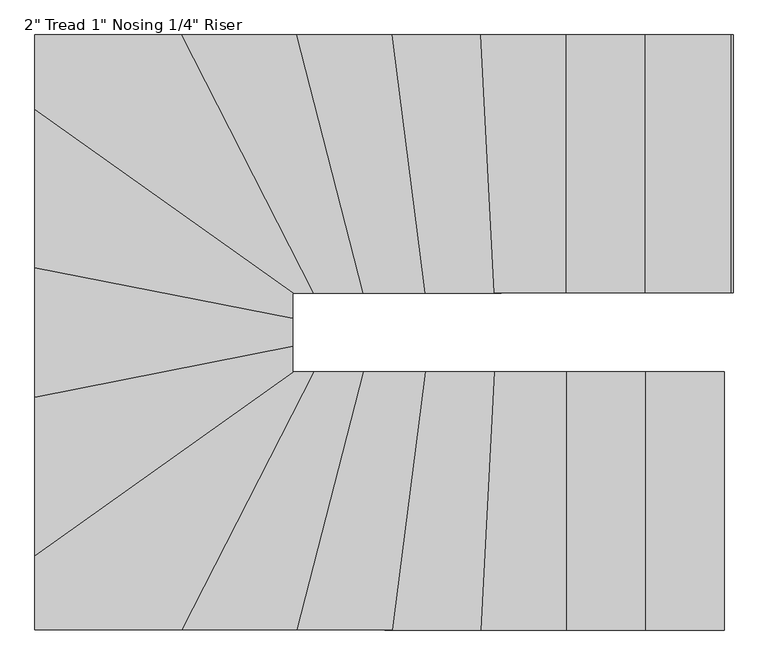
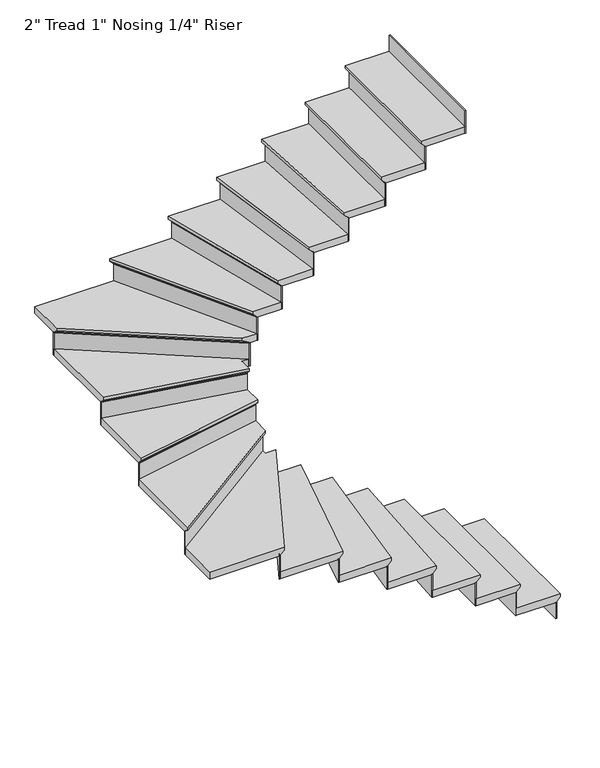
"""IFC4 building model written with IfcOpenShell, lengths in millimetres: stair flight geometry."""

from ifc_helpers import new_model, si_unit, origin, place, context, project, spatial, faceted_brep, source, transform, mapped, element, save


def stair_flight_6e6a5ea5(model_context):
    return source(origin(), model_context, "Body", "Brep", [
        faceted_brep([(-1660.1449167, -345.7070853, 150.2833333), (-1660.1449167, -345.7070853, 169.3333333), (-1660.1449167, -1260.1070853, 169.3333333), (-1660.1449167, -1260.1070853, 150.2833333), (-1685.5449167, -345.7070853, 124.8833333), (-1685.5449167, -1260.1070853, 124.8833333), (-1964.9449167, -345.7070853, 169.3333333), (-1964.9449167, -1260.1070853, 169.3333333), (-1685.5449167, -1260.1070853, 118.5333333), (-1964.9449167, -1260.1070853, 118.5333333), (-1964.9449167, -345.7070853, 118.5333333), (-1685.5449167, -345.7070853, 118.5333333)], [[[0, 1, 2, 3]], [[4, 0, 3, 5]], [[2, 1, 6, 7]], [[8, 9, 10, 11]], [[2, 7, 9, 8, 5, 3]], [[8, 11, 4, 5]], [[6, 1, 0, 4, 11, 10]], [[7, 6, 10, 9]]]),
        faceted_brep([(-1685.5449167, -345.7070853, 118.5333333), (-1685.5449167, -345.7070853, 0.0), (-1691.8949167, -345.7070853, 0.0), (-1691.8949167, -345.7070853, 118.5333333), (-1685.5449167, -1260.1070853, 118.5333333), (-1691.8949167, -1260.1070853, 118.5333333), (-1691.8949167, -1260.1070853, 0.0), (-1685.5449167, -1260.1070853, 0.0)], [[[0, 1, 2, 3]], [[4, 5, 6, 7]], [[1, 0, 4, 7]], [[2, 1, 7, 6]], [[3, 2, 6, 5]], [[0, 3, 5, 4]]]),
        faceted_brep([(-1964.9449167, -345.7070853, 287.8666667), (-1964.9449167, -345.7070853, 118.5333333), (-1971.2949167, -345.7070853, 118.5333333), (-1971.2949167, -345.7070853, 287.8666667), (-1964.9449167, -1260.1070853, 287.8666667), (-1971.2949167, -1260.1070853, 287.8666667), (-1971.2949167, -1260.1070853, 118.5333333), (-1964.9449167, -1260.1070853, 118.5333333)], [[[0, 1, 2, 3]], [[4, 5, 6, 7]], [[1, 0, 4, 7]], [[2, 1, 7, 6]], [[3, 2, 6, 5]], [[0, 3, 5, 4]]]),
        faceted_brep([(-1939.5449167, -1260.1070853, 338.6666667), (-1939.5449167, -345.7070853, 338.6666667), (-2244.3449167, -345.7070853, 338.6666667), (-2244.3449167, -1260.1070853, 338.6666667), (-1964.9449167, -1260.1070853, 287.8666667), (-2244.3449167, -1260.1070853, 287.8666667), (-2244.3449167, -345.7070853, 287.8666667), (-1964.9449167, -345.7070853, 287.8666667), (-1964.9449167, -1260.1070853, 294.2166667), (-1939.5449167, -1260.1070853, 319.6166667), (-1964.9449167, -345.7070853, 294.2166667), (-1939.5449167, -345.7070853, 319.6166667)], [[[0, 1, 2, 3]], [[4, 5, 6, 7]], [[0, 3, 5, 4, 8, 9]], [[4, 7, 10, 8]], [[2, 1, 11, 10, 7, 6]], [[3, 2, 6, 5]], [[11, 1, 0, 9]], [[10, 11, 9, 8]]]),
        faceted_brep([(-2244.3449167, -345.7070853, 457.2), (-2244.3449167, -345.7070853, 287.8666667), (-2250.6949167, -345.7070853, 287.8666667), (-2250.6949167, -345.7070853, 457.2), (-2244.3449167, -1260.1070853, 457.2), (-2250.6949167, -1260.1070853, 457.2), (-2250.6949167, -1260.1070853, 287.8666667), (-2244.3449167, -1260.1070853, 287.8666667)], [[[0, 1, 2, 3]], [[4, 5, 6, 7]], [[1, 0, 4, 7]], [[2, 1, 7, 6]], [[3, 2, 6, 5]], [[0, 3, 5, 4]]]),
        faceted_brep([(-2218.9449167, -1260.1070853, 508.0), (-2218.9449167, -345.7070853, 508.0), (-2500.0120781, -345.7070853, 508.0), (-2547.5463485, -1260.1070853, 508.0), (-2244.3449167, -1260.1070853, 457.2), (-2547.5463485, -1260.1070853, 457.2), (-2500.0120781, -345.7070853, 457.2), (-2244.3449167, -345.7070853, 457.2), (-2244.3449167, -1260.1070853, 463.55), (-2218.9449167, -1260.1070853, 488.95), (-2244.3449167, -345.7070853, 463.55), (-2218.9449167, -345.7070853, 488.95)], [[[0, 1, 2, 3]], [[4, 5, 6, 7]], [[0, 3, 5, 4, 8, 9]], [[4, 7, 10, 8]], [[2, 1, 11, 10, 7, 6]], [[3, 2, 6, 5]], [[11, 1, 0, 9]], [[10, 11, 9, 8]]]),
        faceted_brep([(-2500.0120781, -345.7070853, 626.5333333), (-2500.0120781, -345.7070853, 457.2), (-2506.3706523, -345.7070853, 457.2), (-2506.3706523, -345.7070853, 626.5333333), (-2547.5463485, -1260.1070853, 626.5333333), (-2553.9049227, -1260.1070853, 626.5333333), (-2553.9049227, -1260.1070853, 457.2), (-2547.5463485, -1260.1070853, 457.2)], [[[0, 1, 2, 3]], [[4, 5, 6, 7]], [[1, 0, 4, 7]], [[2, 1, 7, 6]], [[3, 2, 6, 5]], [[0, 3, 5, 4]]]),
        faceted_brep([(-2522.1120519, -1260.1070853, 677.3333333), (-2474.5777815, -345.7070853, 677.3333333), (-2744.178778, -345.7070853, 677.3333333), (-2862.5348296, -1260.1070853, 677.3333333), (-2547.5463485, -1260.1070853, 626.5333333), (-2862.5348296, -1260.1070853, 626.5333333), (-2744.178778, -345.7070853, 626.5333333), (-2500.0120781, -345.7070853, 626.5333333), (-2547.5463485, -1260.1070853, 632.8833333), (-2522.1120519, -1260.1070853, 658.2833333), (-2500.0120781, -345.7070853, 632.8833333), (-2474.5777815, -345.7070853, 658.2833333)], [[[0, 1, 2, 3]], [[4, 5, 6, 7]], [[0, 3, 5, 4, 8, 9]], [[4, 7, 10, 8]], [[2, 1, 11, 10, 7, 6]], [[3, 2, 6, 5]], [[11, 1, 0, 9]], [[10, 11, 9, 8]]]),
        faceted_brep([(-2744.178778, -345.7070853, 795.8666667), (-2744.178778, -345.7070853, 626.5333333), (-2750.5817497, -345.7070853, 626.5333333), (-2750.5817497, -345.7070853, 795.8666667), (-2862.5348296, -1260.1070853, 795.8666667), (-2868.9378014, -1260.1070853, 795.8666667), (-2868.9378014, -1260.1070853, 626.5333333), (-2862.5348296, -1260.1070853, 626.5333333)], [[[0, 1, 2, 3]], [[4, 5, 6, 7]], [[1, 0, 4, 7]], [[2, 1, 7, 6]], [[3, 2, 6, 5]], [[0, 3, 5, 4]]]),
        faceted_brep([(-2836.9229425, -1260.1070853, 846.6666667), (-2718.5668908, -345.7070853, 846.6666667), (-2965.8060004, -345.7070853, 846.6666667), (-3200.9364478, -1260.1070853, 846.6666667), (-2862.5348296, -1260.1070853, 795.8666667), (-3200.9364478, -1260.1070853, 795.8666667), (-2965.8060004, -345.7070853, 795.8666667), (-2744.178778, -345.7070853, 795.8666667), (-2862.5348296, -1260.1070853, 802.2166667), (-2836.9229425, -1260.1070853, 827.6166667), (-2744.178778, -345.7070853, 802.2166667), (-2718.5668908, -345.7070853, 827.6166667)], [[[0, 1, 2, 3]], [[4, 5, 6, 7]], [[0, 3, 5, 4, 8, 9]], [[4, 7, 10, 8]], [[2, 1, 11, 10, 7, 6]], [[3, 2, 6, 5]], [[11, 1, 0, 9]], [[10, 11, 9, 8]]]),
        faceted_brep([(-2965.8060004, -345.7070853, 965.2), (-2965.8060004, -345.7070853, 795.8666667), (-2972.3625773, -345.7070853, 795.8666667), (-2972.3625773, -345.7070853, 965.2), (-3200.9364478, -1260.1070853, 965.2), (-3207.4930247, -1260.1070853, 965.2), (-3207.4930247, -1260.1070853, 795.8666667), (-3200.9364478, -1260.1070853, 795.8666667)], [[[0, 1, 2, 3]], [[4, 5, 6, 7]], [[1, 0, 4, 7]], [[2, 1, 7, 6]], [[3, 2, 6, 5]], [[0, 3, 5, 4]]]),
        faceted_brep([(-3174.7101404, -1260.1070853, 1016.0), (-2939.579693, -345.7070853, 1016.0), (-3142.1526365, -345.7070853, 1016.0), (-3610.9772578, -1260.1070853, 1016.0), (-3200.9364478, -1260.1070853, 965.2), (-3610.9772578, -1260.1070853, 965.2), (-3142.1526365, -345.7070853, 965.2), (-2965.8060004, -345.7070853, 965.2), (-3200.9364478, -1260.1070853, 971.55), (-3174.7101404, -1260.1070853, 996.95), (-2965.8060004, -345.7070853, 971.55), (-2939.579693, -345.7070853, 996.95)], [[[0, 1, 2, 3]], [[4, 5, 6, 7]], [[0, 3, 5, 4, 8, 9]], [[4, 7, 10, 8]], [[2, 1, 11, 10, 7, 6]], [[3, 2, 6, 5]], [[11, 1, 0, 9]], [[10, 11, 9, 8]]]),
        faceted_brep([(-3142.1526365, -345.7070853, 1134.5333333), (-3142.1526365, -345.7070853, 965.2), (-3149.2886197, -345.7070853, 965.2), (-3149.2886197, -345.7070853, 1134.5333333), (-3610.9772578, -1260.1070853, 1134.5333333), (-3618.113241, -1260.1070853, 1134.5333333), (-3618.113241, -1260.1070853, 965.2), (-3610.9772578, -1260.1070853, 965.2)], [[[0, 1, 2, 3]], [[4, 5, 6, 7]], [[1, 0, 4, 7]], [[2, 1, 7, 6]], [[3, 2, 6, 5]], [[0, 3, 5, 4]]]),
        faceted_brep([(-4102.2766085, -966.4259516, 1185.3333333), (-4102.2766085, -1260.1070853, 1185.3333333), (-3582.4333253, -1260.1070853, 1185.3333333), (-3113.608704, -345.7070853, 1185.3333333), (-3187.8766085, -345.7070853, 1185.3333333), (-3187.8766085, -316.1520025, 1185.3333333), (-4102.2766085, -1260.1070853, 1134.5333333), (-4102.2766085, -966.4259516, 1134.5333333), (-3187.8766085, -316.1520025, 1134.5333333), (-3187.8766085, -345.7070853, 1134.5333333), (-3142.1526365, -345.7070853, 1134.5333333), (-3610.9772578, -1260.1070853, 1134.5333333), (-3610.9772578, -1260.1070853, 1140.8833333), (-3582.4333253, -1260.1070853, 1166.2833333), (-3142.1526365, -345.7070853, 1140.8833333), (-3113.608704, -345.7070853, 1166.2833333)], [[[0, 1, 2, 3, 4, 5]], [[6, 7, 8, 9, 10, 11]], [[1, 0, 7, 6]], [[2, 1, 6, 11, 12, 13]], [[11, 10, 14, 12]], [[4, 3, 15, 14, 10, 9]], [[5, 4, 9, 8]], [[0, 5, 8, 7]], [[15, 3, 2, 13]], [[14, 15, 13, 12]]]),
        faceted_brep([(-3187.8766085, -316.1520025, 1303.8666667), (-3187.8766085, -316.1520025, 1134.5333333), (-3187.8766085, -308.3600277, 1134.5333333), (-3187.8766085, -308.3600277, 1303.8666667), (-4102.2766085, -966.4259516, 1303.8666667), (-4102.2766085, -958.6339768, 1303.8666667), (-4102.2766085, -958.6339768, 1134.5333333), (-4102.2766085, -966.4259516, 1134.5333333)], [[[0, 1, 2, 3]], [[4, 5, 6, 7]], [[1, 0, 4, 7]], [[2, 1, 7, 6]], [[3, 2, 6, 5]], [[0, 3, 5, 4]]]),
        faceted_brep([(-4102.2766085, -997.5938508, 1354.6666667), (-3187.8766085, -347.3199017, 1354.6666667), (-3187.8766085, -229.6979154, 1354.6666667), (-4102.2766085, -409.9387717, 1354.6666667), (-4102.2766085, -966.4259516, 1303.8666667), (-4102.2766085, -409.9387717, 1303.8666667), (-3187.8766085, -229.6979154, 1303.8666667), (-3187.8766085, -316.1520025, 1303.8666667), (-4102.2766085, -966.4259516, 1310.2166667), (-4102.2766085, -997.5938508, 1335.6166667), (-3187.8766085, -316.1520025, 1310.2166667), (-3187.8766085, -347.3199017, 1335.6166667)], [[[0, 1, 2, 3]], [[4, 5, 6, 7]], [[0, 3, 5, 4, 8, 9]], [[4, 7, 10, 8]], [[2, 1, 11, 10, 7, 6]], [[3, 2, 6, 5]], [[11, 1, 0, 9]], [[10, 11, 9, 8]]]),
        faceted_brep([(-3187.8766085, -229.6979154, 1473.2), (-3187.8766085, -229.6979154, 1303.8666667), (-3187.8766085, -223.22573, 1303.8666667), (-3187.8766085, -223.22573, 1473.2), (-4102.2766085, -409.9387717, 1473.2), (-4102.2766085, -403.4665863, 1473.2), (-4102.2766085, -403.4665863, 1303.8666667), (-4102.2766085, -409.9387717, 1303.8666667)], [[[0, 1, 2, 3]], [[4, 5, 6, 7]], [[1, 0, 4, 7]], [[2, 1, 7, 6]], [[3, 2, 6, 5]], [[0, 3, 5, 4]]]),
        faceted_brep([(-4102.2766085, -435.8275135, 1524.0), (-3187.8766085, -255.5866572, 1524.0), (-3187.8766085, -130.5387717, 1524.0), (-4102.2766085, 49.7020846, 1524.0), (-4102.2766085, -409.9387717, 1473.2), (-4102.2766085, 49.7020846, 1473.2), (-3187.8766085, -130.5387717, 1473.2), (-3187.8766085, -229.6979154, 1473.2), (-4102.2766085, -409.9387717, 1479.55), (-4102.2766085, -435.8275135, 1504.95), (-3187.8766085, -229.6979154, 1479.55), (-3187.8766085, -255.5866572, 1504.95)], [[[0, 1, 2, 3]], [[4, 5, 6, 7]], [[0, 3, 5, 4, 8, 9]], [[4, 7, 10, 8]], [[2, 1, 11, 10, 7, 6]], [[3, 2, 6, 5]], [[11, 1, 0, 9]], [[10, 11, 9, 8]]]),
        faceted_brep([(-3187.8766085, -130.5387717, 1642.5333333), (-3187.8766085, -130.5387717, 1473.2), (-3187.8766085, -124.0665863, 1473.2), (-3187.8766085, -124.0665863, 1642.5333333), (-4102.2766085, 49.7020846, 1642.5333333), (-4102.2766085, 56.17427, 1642.5333333), (-4102.2766085, 56.17427, 1473.2), (-4102.2766085, 49.7020846, 1473.2)], [[[0, 1, 2, 3]], [[4, 5, 6, 7]], [[1, 0, 4, 7]], [[2, 1, 7, 6]], [[3, 2, 6, 5]], [[0, 3, 5, 4]]]),
        faceted_brep([(-4102.2766085, 23.8133428, 1693.3333333), (-3187.8766085, -156.4275135, 1693.3333333), (-3187.8766085, -66.3070853, 1693.3333333), (-3141.781134, -66.3070853, 1693.3333333), (-4102.2766085, 616.7475793, 1693.3333333), (-4102.2766085, 49.7020846, 1642.5333333), (-4102.2766085, 616.7475793, 1642.5333333), (-3141.781134, -66.3070853, 1642.5333333), (-3187.8766085, -66.3070853, 1642.5333333), (-3187.8766085, -130.5387717, 1642.5333333), (-4102.2766085, 49.7020846, 1648.8833333), (-4102.2766085, 23.8133428, 1674.2833333), (-3187.8766085, -130.5387717, 1648.8833333), (-3187.8766085, -156.4275135, 1674.2833333)], [[[0, 1, 2, 3, 4]], [[5, 6, 7, 8, 9]], [[0, 4, 6, 5, 10, 11]], [[5, 9, 12, 10]], [[2, 1, 13, 12, 9, 8]], [[3, 2, 8, 7]], [[4, 3, 7, 6]], [[13, 1, 0, 11]], [[12, 13, 11, 10]]]),
        faceted_brep([(-3141.781134, -66.3070853, 1811.8666667), (-3141.781134, -66.3070853, 1642.5333333), (-3130.8242415, -66.3070853, 1642.5333333), (-3130.8242415, -66.3070853, 1811.8666667), (-4102.2766085, 616.7475793, 1811.8666667), (-4102.2766085, 624.5395541, 1811.8666667), (-4102.2766085, 624.5395541, 1642.5333333), (-4102.2766085, 616.7475793, 1642.5333333)], [[[0, 1, 2, 3]], [[4, 5, 6, 7]], [[1, 0, 4, 7]], [[2, 1, 7, 6]], [[3, 2, 6, 5]], [[0, 3, 5, 4]]]),
        faceted_brep([(-3553.8893928, 848.0929147, 1862.6666667), (-4102.2766085, 848.0929147, 1862.6666667), (-4102.2766085, 585.5796802, 1862.6666667), (-3185.608704, -66.3070853, 1862.6666667), (-3085.0647715, -66.3070853, 1862.6666667), (-4102.2766085, 848.0929147, 1811.8666667), (-3553.8893928, 848.0929147, 1811.8666667), (-3085.0647715, -66.3070853, 1811.8666667), (-3141.781134, -66.3070853, 1811.8666667), (-4102.2766085, 616.7475793, 1811.8666667), (-4102.2766085, 616.7475793, 1818.2166667), (-4102.2766085, 585.5796802, 1843.6166667), (-3141.781134, -66.3070853, 1818.2166667), (-3185.608704, -66.3070853, 1843.6166667)], [[[0, 1, 2, 3, 4]], [[5, 6, 7, 8, 9]], [[1, 0, 6, 5]], [[2, 1, 5, 9, 10, 11]], [[9, 8, 12, 10]], [[4, 3, 13, 12, 8, 7]], [[0, 4, 7, 6]], [[13, 3, 2, 11]], [[12, 13, 11, 10]]]),
        faceted_brep([(-3085.0647715, -66.3070853, 1981.2), (-3085.0647715, -66.3070853, 1811.8666667), (-3077.9287883, -66.3070853, 1811.8666667), (-3077.9287883, -66.3070853, 1981.2), (-3553.8893928, 848.0929147, 1981.2), (-3546.7534096, 848.0929147, 1981.2), (-3546.7534096, 848.0929147, 1811.8666667), (-3553.8893928, 848.0929147, 1811.8666667)], [[[0, 1, 2, 3]], [[4, 5, 6, 7]], [[1, 0, 4, 7]], [[2, 1, 7, 6]], [[3, 2, 6, 5]], [[0, 3, 5, 4]]]),
        faceted_brep([(-3582.4333253, 848.0929147, 2032.0), (-3113.608704, -66.3070853, 2032.0), (-2913.3533855, -66.3070853, 2032.0), (-3148.4838329, 848.0929147, 2032.0), (-3553.8893928, 848.0929147, 1981.2), (-3148.4838329, 848.0929147, 1981.2), (-2913.3533855, -66.3070853, 1981.2), (-3085.0647715, -66.3070853, 1981.2), (-3553.8893928, 848.0929147, 1987.55), (-3582.4333253, 848.0929147, 2012.95), (-3085.0647715, -66.3070853, 1987.55), (-3113.608704, -66.3070853, 2012.95)], [[[0, 1, 2, 3]], [[4, 5, 6, 7]], [[0, 3, 5, 4, 8, 9]], [[4, 7, 10, 8]], [[2, 1, 11, 10, 7, 6]], [[3, 2, 6, 5]], [[11, 1, 0, 9]], [[10, 11, 9, 8]]]),
        faceted_brep([(-2913.3533855, -66.3070853, 2150.5333333), (-2913.3533855, -66.3070853, 1981.2), (-2906.7968086, -66.3070853, 1981.2), (-2906.7968086, -66.3070853, 2150.5333333), (-3148.4838329, 848.0929147, 2150.5333333), (-3141.9272561, 848.0929147, 2150.5333333), (-3141.9272561, 848.0929147, 1981.2), (-3148.4838329, 848.0929147, 1981.2)], [[[0, 1, 2, 3]], [[4, 5, 6, 7]], [[1, 0, 4, 7]], [[2, 1, 7, 6]], [[3, 2, 6, 5]], [[0, 3, 5, 4]]]),
        faceted_brep([(-3174.7101404, 848.0929147, 2201.3333333), (-2939.579693, -66.3070853, 2201.3333333), (-2692.9550037, -66.3070853, 2201.3333333), (-2811.3110554, 848.0929147, 2201.3333333), (-3148.4838329, 848.0929147, 2150.5333333), (-2811.3110554, 848.0929147, 2150.5333333), (-2692.9550037, -66.3070853, 2150.5333333), (-2913.3533855, -66.3070853, 2150.5333333), (-3148.4838329, 848.0929147, 2156.8833333), (-3174.7101404, 848.0929147, 2182.2833333), (-2913.3533855, -66.3070853, 2156.8833333), (-2939.579693, -66.3070853, 2182.2833333)], [[[0, 1, 2, 3]], [[4, 5, 6, 7]], [[0, 3, 5, 4, 8, 9]], [[4, 7, 10, 8]], [[2, 1, 11, 10, 7, 6]], [[3, 2, 6, 5]], [[11, 1, 0, 9]], [[10, 11, 9, 8]]]),
        faceted_brep([(-2692.9550037, -66.3070853, 2319.8666667), (-2692.9550037, -66.3070853, 2150.5333333), (-2686.552032, -66.3070853, 2150.5333333), (-2686.552032, -66.3070853, 2319.8666667), (-2811.3110554, 848.0929147, 2319.8666667), (-2804.9080836, 848.0929147, 2319.8666667), (-2804.9080836, 848.0929147, 2150.5333333), (-2811.3110554, 848.0929147, 2150.5333333)], [[[0, 1, 2, 3]], [[4, 5, 6, 7]], [[1, 0, 4, 7]], [[2, 1, 7, 6]], [[3, 2, 6, 5]], [[0, 3, 5, 4]]]),
        faceted_brep([(-2836.9229425, 848.0929147, 2370.6666667), (-2718.5668908, -66.3070853, 2370.6666667), (-2449.1434848, -66.3070853, 2370.6666667), (-2496.6777552, 848.0929147, 2370.6666667), (-2811.3110554, 848.0929147, 2319.8666667), (-2496.6777552, 848.0929147, 2319.8666667), (-2449.1434848, -66.3070853, 2319.8666667), (-2692.9550037, -66.3070853, 2319.8666667), (-2811.3110554, 848.0929147, 2326.2166667), (-2836.9229425, 848.0929147, 2351.6166667), (-2692.9550037, -66.3070853, 2326.2166667), (-2718.5668908, -66.3070853, 2351.6166667)], [[[0, 1, 2, 3]], [[4, 5, 6, 7]], [[0, 3, 5, 4, 8, 9]], [[4, 7, 10, 8]], [[2, 1, 11, 10, 7, 6]], [[3, 2, 6, 5]], [[11, 1, 0, 9]], [[10, 11, 9, 8]]]),
        faceted_brep([(-2449.1434848, -66.3070853, 2489.2), (-2449.1434848, -66.3070853, 2319.8666667), (-2442.7849106, -66.3070853, 2319.8666667), (-2442.7849106, -66.3070853, 2489.2), (-2496.6777552, 848.0929147, 2489.2), (-2490.3191811, 848.0929147, 2489.2), (-2490.3191811, 848.0929147, 2319.8666667), (-2496.6777552, 848.0929147, 2319.8666667)], [[[0, 1, 2, 3]], [[4, 5, 6, 7]], [[1, 0, 4, 7]], [[2, 1, 7, 6]], [[3, 2, 6, 5]], [[0, 3, 5, 4]]]),
        faceted_brep([(-2522.1120519, 848.0929147, 2540.0), (-2474.5777815, -66.3070853, 2540.0), (-2193.5449167, -66.3070853, 2540.0), (-2193.5449167, 848.0929147, 2540.0), (-2496.6777552, 848.0929147, 2489.2), (-2193.5449167, 848.0929147, 2489.2), (-2193.5449167, -66.3070853, 2489.2), (-2449.1434848, -66.3070853, 2489.2), (-2496.6777552, 848.0929147, 2495.55), (-2522.1120519, 848.0929147, 2520.95), (-2449.1434848, -66.3070853, 2495.55), (-2474.5777815, -66.3070853, 2520.95)], [[[0, 1, 2, 3]], [[4, 5, 6, 7]], [[0, 3, 5, 4, 8, 9]], [[4, 7, 10, 8]], [[2, 1, 11, 10, 7, 6]], [[3, 2, 6, 5]], [[11, 1, 0, 9]], [[10, 11, 9, 8]]]),
        faceted_brep([(-2193.5449167, -66.3070853, 2658.5333333), (-2193.5449167, -66.3070853, 2489.2), (-2187.1949167, -66.3070853, 2489.2), (-2187.1949167, -66.3070853, 2658.5333333), (-2193.5449167, 848.0929147, 2658.5333333), (-2187.1949167, 848.0929147, 2658.5333333), (-2187.1949167, 848.0929147, 2489.2), (-2193.5449167, 848.0929147, 2489.2)], [[[0, 1, 2, 3]], [[4, 5, 6, 7]], [[1, 0, 4, 7]], [[2, 1, 7, 6]], [[3, 2, 6, 5]], [[0, 3, 5, 4]]]),
        faceted_brep([(-2218.9449167, 848.0929147, 2709.3333333), (-2218.9449167, -66.3070853, 2709.3333333), (-1914.1449167, -66.3070853, 2709.3333333), (-1914.1449167, 848.0929147, 2709.3333333), (-2193.5449167, 848.0929147, 2658.5333333), (-1914.1449167, 848.0929147, 2658.5333333), (-1914.1449167, -66.3070853, 2658.5333333), (-2193.5449167, -66.3070853, 2658.5333333), (-2193.5449167, 848.0929147, 2664.8833333), (-2218.9449167, 848.0929147, 2690.2833333), (-2193.5449167, -66.3070853, 2664.8833333), (-2218.9449167, -66.3070853, 2690.2833333)], [[[0, 1, 2, 3]], [[4, 5, 6, 7]], [[0, 3, 5, 4, 8, 9]], [[4, 7, 10, 8]], [[2, 1, 11, 10, 7, 6]], [[3, 2, 6, 5]], [[11, 1, 0, 9]], [[10, 11, 9, 8]]]),
        faceted_brep([(-1914.1449167, -66.3070853, 2827.8666667), (-1914.1449167, -66.3070853, 2658.5333333), (-1907.7949167, -66.3070853, 2658.5333333), (-1907.7949167, -66.3070853, 2827.8666667), (-1914.1449167, 848.0929147, 2827.8666667), (-1907.7949167, 848.0929147, 2827.8666667), (-1907.7949167, 848.0929147, 2658.5333333), (-1914.1449167, 848.0929147, 2658.5333333)], [[[0, 1, 2, 3]], [[4, 5, 6, 7]], [[1, 0, 4, 7]], [[2, 1, 7, 6]], [[3, 2, 6, 5]], [[0, 3, 5, 4]]]),
        faceted_brep([(-1634.7449167, -66.3070853, 2997.2), (-1634.7449167, -66.3070853, 2827.8666667), (-1628.3949167, -66.3070853, 2827.8666667), (-1628.3949167, -66.3070853, 2997.2), (-1634.7449167, 848.0929147, 2997.2), (-1628.3949167, 848.0929147, 2997.2), (-1628.3949167, 848.0929147, 2827.8666667), (-1634.7449167, 848.0929147, 2827.8666667)], [[[0, 1, 2, 3]], [[4, 5, 6, 7]], [[1, 0, 4, 7]], [[2, 1, 7, 6]], [[3, 2, 6, 5]], [[0, 3, 5, 4]]]),
        faceted_brep([(-1939.5449167, 848.0929147, 2878.6666667), (-1939.5449167, -66.3070853, 2878.6666667), (-1634.7449167, -66.3070853, 2878.6666667), (-1634.7449167, 848.0929147, 2878.6666667), (-1914.1449167, 848.0929147, 2827.8666667), (-1634.7449167, 848.0929147, 2827.8666667), (-1634.7449167, -66.3070853, 2827.8666667), (-1914.1449167, -66.3070853, 2827.8666667), (-1914.1449167, 848.0929147, 2834.2166667), (-1939.5449167, 848.0929147, 2859.6166667), (-1914.1449167, -66.3070853, 2834.2166667), (-1939.5449167, -66.3070853, 2859.6166667)], [[[0, 1, 2, 3]], [[4, 5, 6, 7]], [[0, 3, 5, 4, 8, 9]], [[4, 7, 10, 8]], [[2, 1, 11, 10, 7, 6]], [[3, 2, 6, 5]], [[11, 1, 0, 9]], [[10, 11, 9, 8]]]),
    ])


if __name__ == "__main__":
    model = new_model("IFC4")
    model_context = context("Model", 3, world=origin())
    ifc_project = project(units=[si_unit("LENGTHUNIT", "METRE", prefix="MILLI")], contexts=[model_context])
    site = spatial("IfcSite", under=ifc_project)
    building = spatial("IfcBuilding", under=site)
    placement = place(None, origin())
    stair_flight_shape = stair_flight_6e6a5ea5(model_context)
    element("IfcStairFlight", 1, ObjectType="2\" Tread 1\" Nosing 1/4\" Riser", at=placement, inside=building, context=model_context, shape_type="MappedRepresentation", body=[
        mapped(stair_flight_shape, transform((0.0, 0.0, 0.0), x_axis=(1.0, 0.0, 0.0), y_axis=(0.0, 1.0, 0.0), z_axis=(0.0, 0.0, 1.0))),
    ])
    save(model, "model.ifc")
